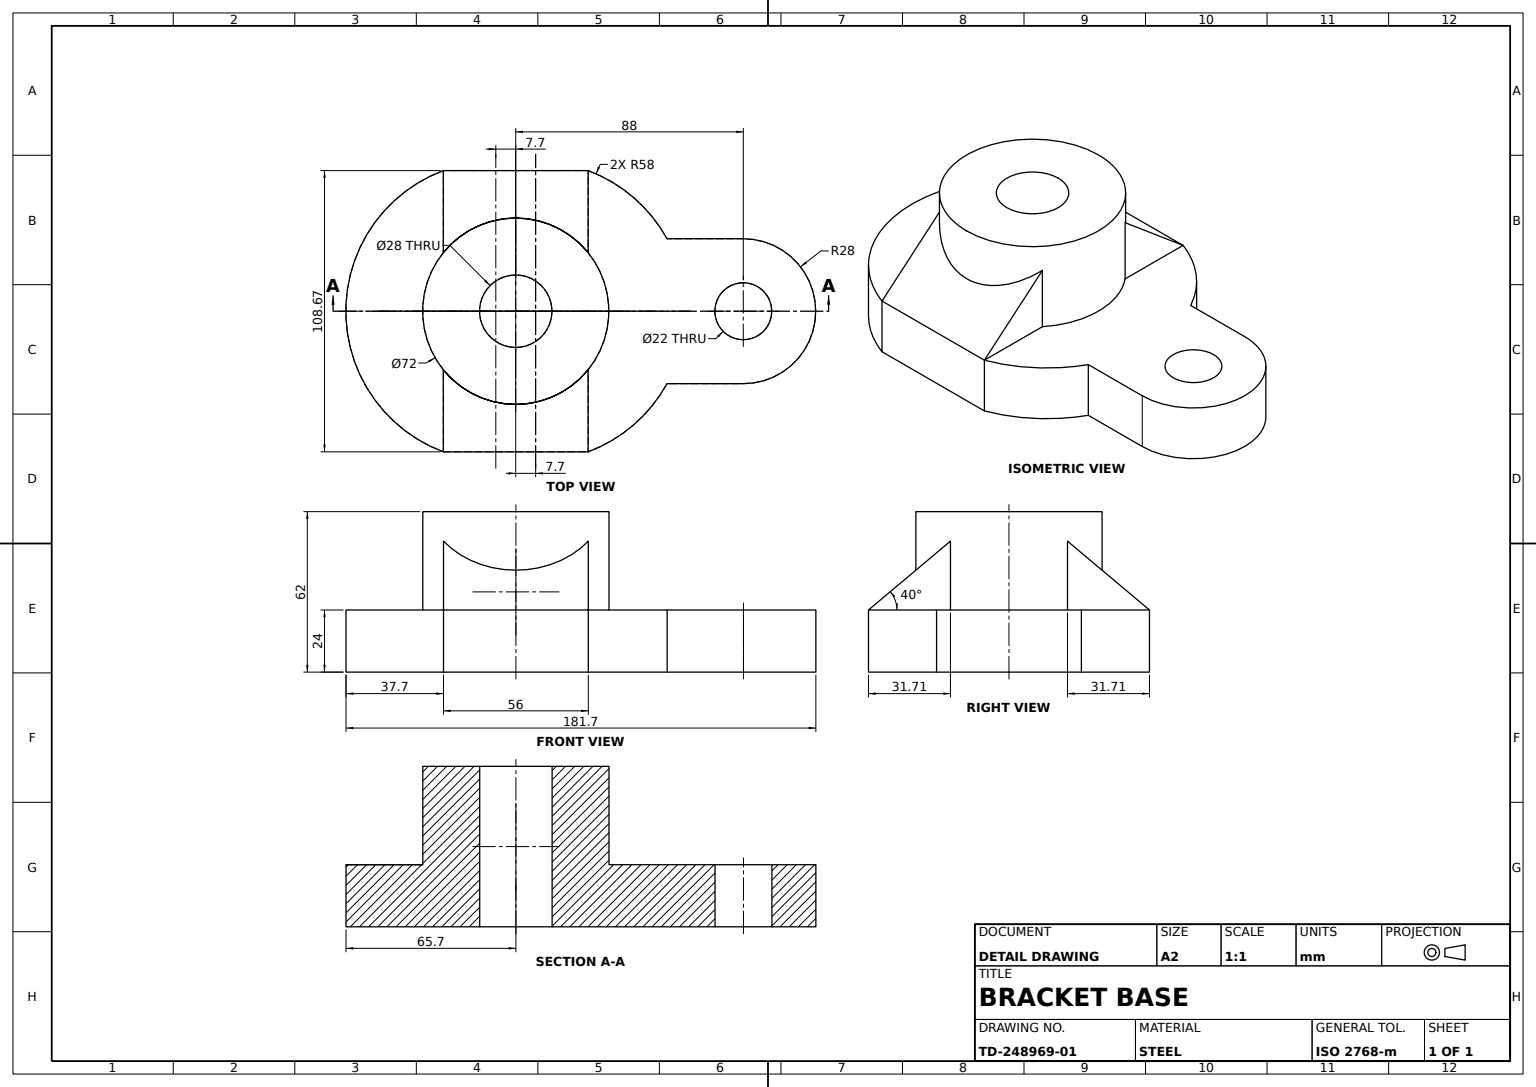
SolidWorks part; units mm, degrees
material "Plain Carbon Steel"
ref_plane "Front Plane" through (0, 0, 0) normal (0, 0, 1) x (1, 0, 0)
ref_plane "Top Plane" through (0, 0, 0) normal (0, 1, 0) x (1, 0, 0)
ref_plane "Right Plane" through (0, 0, 0) normal (1, 0, 0) x (0, 0, -1)
sketch "Base Flange Sketch" plane through (0, 0, 0) normal (0, 1, 0) x (1, 0, 0)
  line L0 (0, 0) -> (-88, 0) construction
  line L1 (-116, 54.3328) -> (-60, 54.3328)
  line L2 (-116, -54.3328) -> (-60, -54.3328)
  line L3 (0, 28) -> (-29.5028, 28)
  line L4 (0, -28) -> (-29.5028, -28)
  line L5 (-88, 0) -> (-88, 24.1265) construction
  arc A0 (0, -28) -> (0, 28) centre (0, 0) ccw
  circle A1 centre (0, 0) radius 11
  arc A2 (-116, -54.3328) -> (-116, 54.3328) centre (-95.7035, 0) cw
  arc A3 (-60, 54.3328) -> (-29.5028, 28) centre (-80.2965, 0) cw
  arc A4 (-29.5028, -28) -> (-60, -54.3328) centre (-80.2965, 0) cw
  point P8 (-88, 54.3328)
  point P16 (-88, -54.3328)
  point P17 (-153.7035, 0)
  dimension "D1" = 56
  dimension "D2" = 22
  dimension "D5" = 58
  dimension "D6" = 108.6656
  dimension "D7" = 58
  dimension "D3" = 88
  dimension "D4" = 56
extrude "Base Flange" add sketch "Base Flange Sketch" along normal blind 24
sketch "Hub Boss Sketch Ø72" plane through (0, 24, 0) normal (0, 1, 0) x (1, 0, 0)
  line L0 (-60, 54.3328) -> (-116, 54.3328) construction
  circle A0 centre (-88, 0) radius 36
  point P5 (-88, 54.3328)
  dimension "D1" = 72
extrude "Hub Boss Ø72" add sketch "Hub Boss Sketch Ø72" along normal blind 38
ref_plane "Wedge Support Plane" through (-88, 0, 0) normal (1, 0, 0) x (0, 0, -1)
sketch "Wedge Support Sketch" plane through (-88, 0, 0) normal (1, 0, 0) x (0, 0, -1)
  line L0 (-54.3328, 24) -> (-13.5043, 58.2591)
  line L1 (-28, 24) -> (-54.3328, 24) construction
  line L2 (13.2664, 58.4587) -> (54.3328, 24)
  line L3 (54.3328, 24) -> (28, 24) construction
  line L7 (-54.3328, 24) -> (54.3328, 24)
  line L8 (-13.5043, 58.2591) -> (13.2664, 58.4587)
  dimension "D1" = 40
  dimension "D2" = 40
  dimension "D3" = 40.8285
  dimension "D4" = 67.5992
extrude "Wedge Support" add sketch "Wedge Support Sketch" along normal mid plane 56
sketch "Bore Sketch Ø28" plane through (0, 62, 0) normal (0, 1, 0) x (1, 0, 0)
  circle A0 centre (-88, 0) radius 14
  arc A1 (-60, 22.6274) -> (-116, 22.6274) centre (-88, 0) ccw construction
  dimension "D1" = 28
extrude "Bore Ø28" cut sketch "Bore Sketch Ø28" against normal up to next
